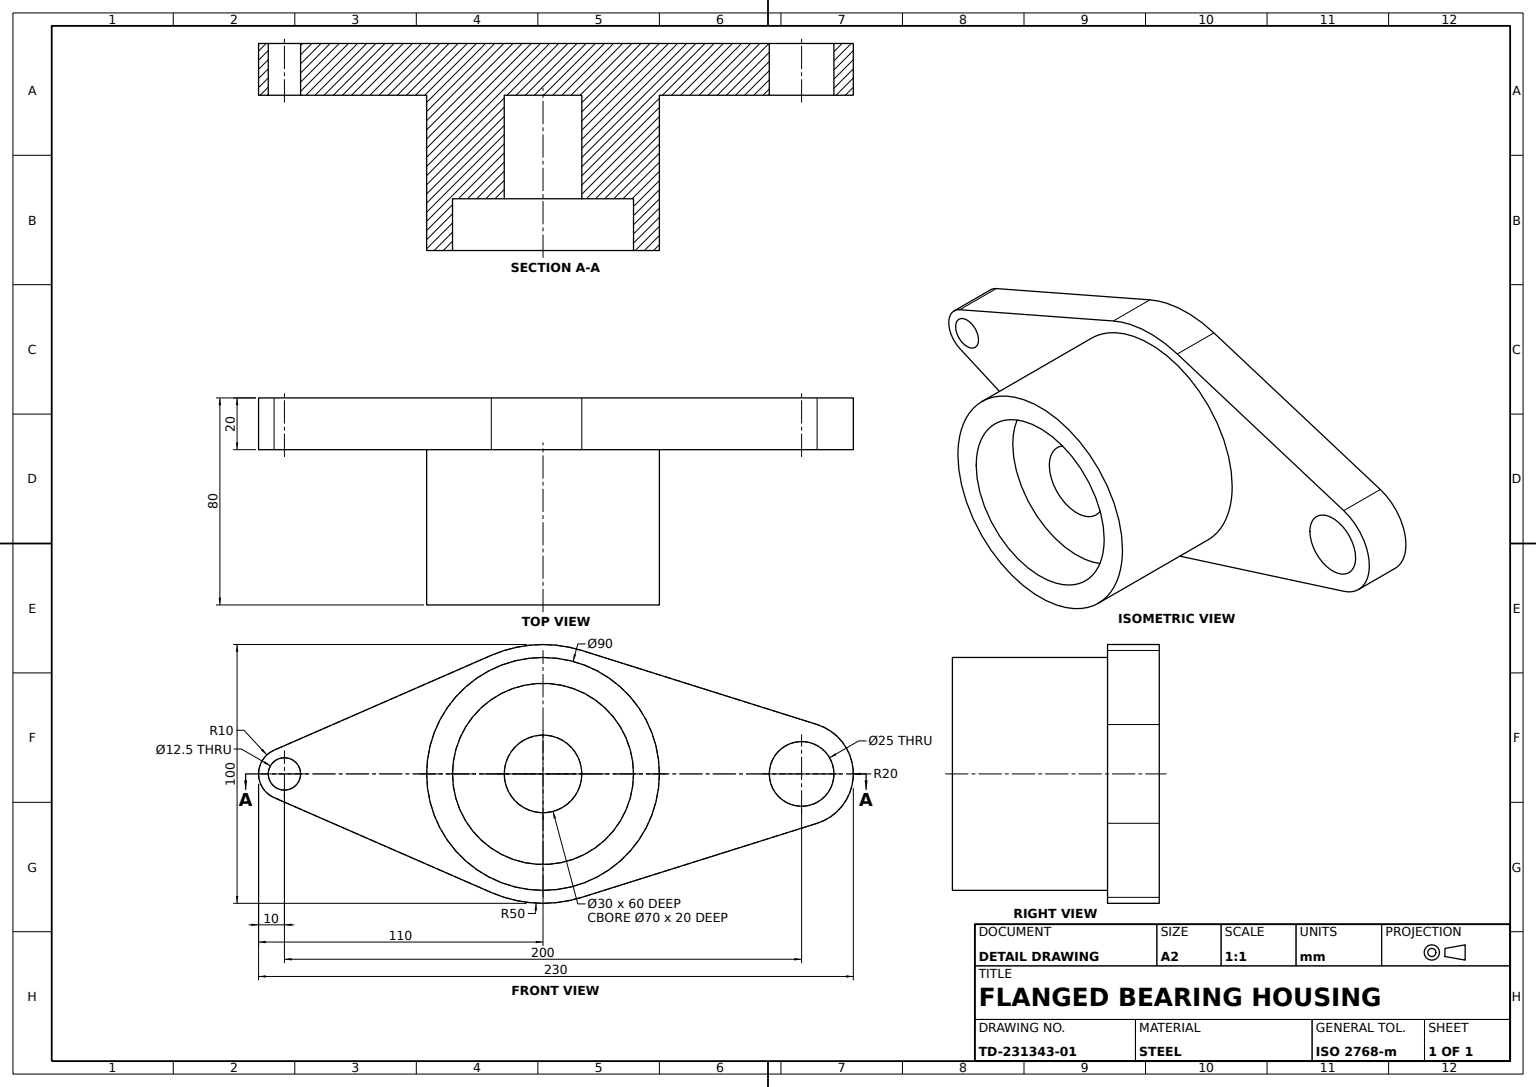
SolidWorks part; units mm, degrees
material "Plain Carbon Steel"
ref_plane "Front Plane" through (0, 0, 0) normal (0, 0, 1) x (1, 0, 0)
ref_plane "Top Plane" through (0, 0, 0) normal (0, 1, 0) x (1, 0, 0)
ref_plane "Right Plane" through (0, 0, 0) normal (1, 0, 0) x (0, 0, -1)
sketch "Flange Plate Profile" plane through (0, 0, 0) normal (0, 0, 1) x (1, 0, 0)
  line L0 (0, 0) -> (100, 0) construction
  line L1 (100, 0) -> (200, 0) construction
  line L2 (-4, 9.1652) -> (80, 45.8258)
  line L3 (-4, -9.1652) -> (80, -45.8258)
  line L4 (115, 47.697) -> (206, 19.0788)
  line L5 (115, -47.697) -> (206, -19.0788)
  circle A0 centre (0, 0) radius 6.25
  arc A1 (-4, 9.1652) -> (-4, -9.1652) centre (0, 0) ccw
  circle A2 centre (200, 0) radius 12.5
  arc A3 (206, -19.0788) -> (206, 19.0788) centre (200, 0) ccw
  arc A4 (80, -45.8258) -> (115, -47.697) centre (100, 0) ccw
  arc A5 (115, 47.697) -> (80, 45.8258) centre (100, 0) ccw
  dimension "D1" = 12.5
  dimension "D2" = 20
  dimension "D3" = 25
  dimension "D4" = 40
  dimension "D6" = 100
  dimension "D5" = 200
  dimension "D7" = 100
extrude "Flange Plate 20mm" add sketch "Flange Plate Profile" along normal blind 20
sketch "Hub Profile Ø90-Ø70" plane through (0, 0, 20) normal (0, 0, 1) x (1, 0, 0)
  circle A0 centre (100, 0) radius 45
  circle A1 centre (100, 0) radius 35
  dimension "D1" = 90
  dimension "D2" = 70
extrude "Hub Ø90x60" add sketch "Hub Profile Ø90-Ø70" along normal blind 60
sketch "Inner Boss Profile Ø70-Ø30" plane through (0, 0, 20) normal (0, 0, 1) x (1, 0, 0)
  circle A0 centre (100, 0) radius 35
  circle A1 centre (100, 0) radius 15
  dimension "D1" = 70
  dimension "D2" = 30
extrude "Inner Boss Ø70 Bore Ø30" add sketch "Inner Boss Profile Ø70-Ø30" along normal blind 40
